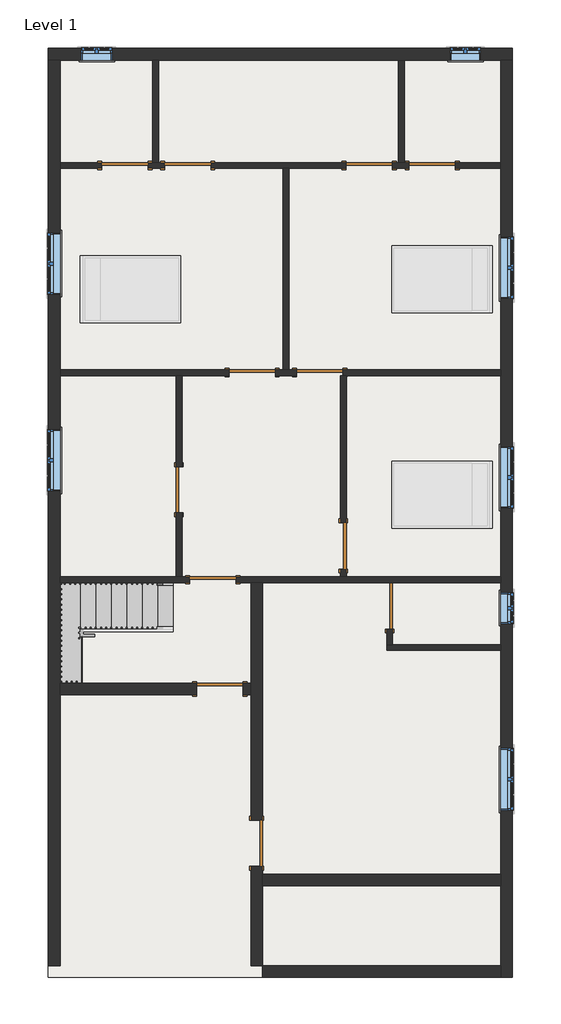
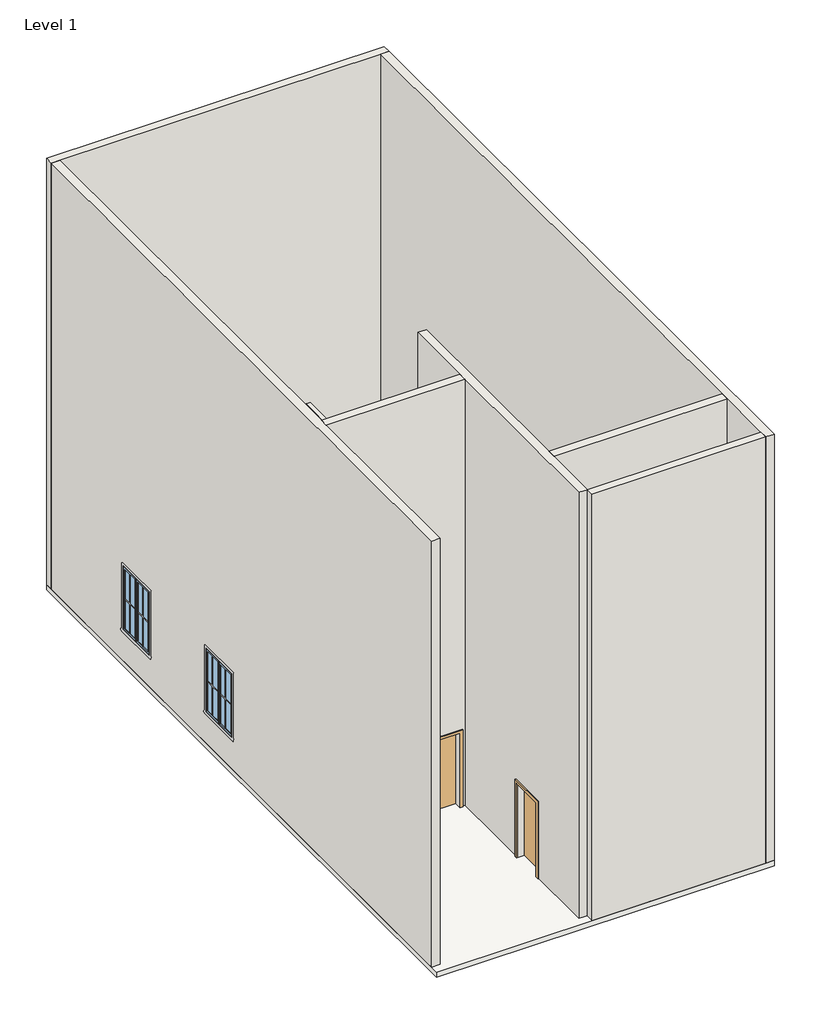
# One storey, part 1 of 2: 17 walls, 12 doors, 8 windows, 1 railing, 1 slab, 1 stair flight.
# Revit data of these elements (continued)
# Element 40 (IfcWindow, "Window-Casement-Double : 48\" x 72\"")
#   Mark = "5"
#   Window Inset = 0' - 0"
#   Interior Wall Closure = 0' - 2 1/4"
#   Frame Extension = 0' - 0 1/4"
#   Exterior Wall Closure = 0' - 1 1/4"
#   Interior Trim Visibility = yes
#   Exterior Trim Visibility = yes
#   Phase Created = New Construction
#   Materials on its faces: "Wood - Stained", "Glass", "Clad - White"
# Materials
#   "Door - Panel": class "Wood", colour RGB 210 159 95, transparency 0, Cost = 0
#   "Door - Frame": colour RGB 118 70 51, transparency 0, Cost = 0
#   "Parking Stripe": class "Paint", colour RGB 250 250 91, transparency 0, Cost = 0
#   "Wood - Stained": class "Wood", colour RGB 224 178 126, transparency 0, Cost = 0
#   "Glass": class "Glass", colour RGB 0 128 192, transparency 0.75, Description = "Soda Lime Glass", Cost = 0
#   "Clad - White": class "Wood", colour RGB 242 242 238, transparency 0, Cost = 0
#   "Default Wall": colour RGB 128 128 128, transparency 0, Cost = 0
